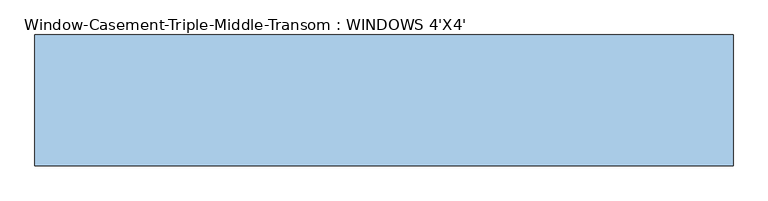
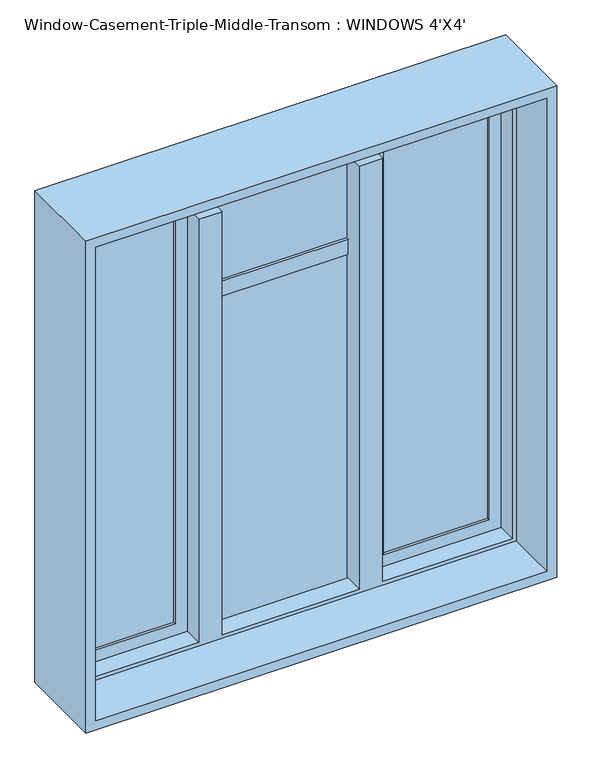
"""IFC4 building model written with IfcOpenShell, lengths in millimetres: window geometry, Window-Casement-Triple-Middle-Transom : WINDOWS 4'X4'."""

from ifc_helpers import new_model, si_unit, frame, origin, place, context, project, spatial, polyline, outline, extrude, faceted_brep, source, transform, mapped, element, save


def window_casement_triple_middle_transom_windows_4_x4_273a115f(model_context):
    return source(origin(), model_context, "Body", "SolidModel", [
        extrude(outline(polyline([(2235.2, 228.6), (939.8, 228.6), (939.8, 584.2), (2235.2, 584.2), (2235.2, 228.6)]), holes=[polyline([(2193.3296875, 542.3296875), (981.6703125, 542.3296875), (981.6703125, 270.4703125), (2193.3296875, 270.4703125), (2193.3296875, 542.3296875)])]), frame((0.0, 73.025, 0.0), z_axis=(0.0, 1.0, 0.0), x_axis=(0.0, 0.0, 1.0)), (0.0, 0.0, 1.0), 31.75),
        extrude(outline(polyline([(2235.2, -584.2), (939.8, -584.2), (939.8, -228.6), (2235.2, -228.6), (2235.2, -584.2)]), holes=[polyline([(2193.3296875, -270.4703125), (981.6703125, -270.4703125), (981.6703125, -542.3296875), (2193.3296875, -542.3296875), (2193.3296875, -270.4703125)])]), frame((0.0, 73.025, 0.0), z_axis=(0.0, 1.0, 0.0), x_axis=(0.0, 0.0, 1.0)), (0.0, 0.0, 1.0), 31.75),
        extrude(outline(polyline([(-270.4703125, 98.425), (-270.4703125, 92.075), (-542.3296875, 92.075), (-542.3296875, 98.425), (-270.4703125, 98.425)])), frame((0.0, 0.0, 949.9203125), z_axis=(0.0, 0.0, 1.0), x_axis=(1.0, 0.0, 0.0)), (0.0, 0.0, 1.0), 1275.159375),
        extrude(outline(polyline([(-270.4703125, 85.725), (-270.4703125, 79.375), (-542.3296875, 79.375), (-542.3296875, 85.725), (-270.4703125, 85.725)])), frame((0.0, 0.0, 949.9203125), z_axis=(0.0, 0.0, 1.0), x_axis=(1.0, 0.0, 0.0)), (0.0, 0.0, 1.0), 1275.159375),
        extrude(outline(polyline([(542.3296875, 98.425), (542.3296875, 92.075), (270.4703125, 92.075), (270.4703125, 98.425), (542.3296875, 98.425)])), frame((0.0, 0.0, 949.9203125), z_axis=(0.0, 0.0, 1.0), x_axis=(1.0, 0.0, 0.0)), (0.0, 0.0, 1.0), 1275.159375),
        extrude(outline(polyline([(542.3296875, 85.725), (542.3296875, 79.375), (270.4703125, 79.375), (270.4703125, 85.725), (542.3296875, 85.725)])), frame((0.0, 0.0, 949.9203125), z_axis=(0.0, 0.0, 1.0), x_axis=(1.0, 0.0, 0.0)), (0.0, 0.0, 1.0), 1275.159375),
        extrude(outline(polyline([(177.8, 104.775), (177.8, 73.025), (-177.8, 73.025), (-177.8, 104.775), (177.8, 104.775)])), frame((0.0, 0.0, 1835.8048438), z_axis=(0.0, 0.0, 1.0), x_axis=(1.0, 0.0, 0.0)), (0.0, 0.0, 1.0), 41.8703125),
        extrude(outline(polyline([(177.8, 98.425), (177.8, 92.075), (-177.8, 92.075), (-177.8, 98.425), (177.8, 98.425)])), frame((0.0, 0.0, 939.8), z_axis=(0.0, 0.0, 1.0), x_axis=(1.0, 0.0, 0.0)), (0.0, 0.0, 1.0), 896.0048437),
        extrude(outline(polyline([(177.8, 85.725), (177.8, 79.375), (-177.8, 79.375), (-177.8, 85.725), (177.8, 85.725)])), frame((0.0, 0.0, 939.8), z_axis=(0.0, 0.0, 1.0), x_axis=(1.0, 0.0, 0.0)), (0.0, 0.0, 1.0), 896.0048437),
        extrude(outline(polyline([(177.8, 98.425), (177.8, 92.075), (-177.8, 92.075), (-177.8, 98.425), (177.8, 98.425)])), frame((0.0, 0.0, 1877.6751563), z_axis=(0.0, 0.0, 1.0), x_axis=(1.0, 0.0, 0.0)), (0.0, 0.0, 1.0), 357.5248438),
        extrude(outline(polyline([(177.8, 85.725), (177.8, 79.375), (-177.8, 79.375), (-177.8, 85.725), (177.8, 85.725)])), frame((0.0, 0.0, 1877.6751563), z_axis=(0.0, 0.0, 1.0), x_axis=(1.0, 0.0, 0.0)), (0.0, 0.0, 1.0), 357.5248438),
        faceted_brep([(-584.2, 73.025, 2235.2), (-584.2, 114.3, 2235.2), (584.2, 114.3, 2235.2), (584.2, 73.025, 2235.2), (-574.0796875, 22.225, 2225.0796875), (-574.0796875, 73.025, 2225.0796875), (574.0796875, 73.025, 2225.0796875), (574.0796875, 22.225, 2225.0796875), (-584.2, -114.3, 2235.2), (-584.2, 22.225, 2235.2), (584.2, 22.225, 2235.2), (584.2, -114.3, 2235.2), (-609.6, 114.3, 2260.6), (-609.6, -114.3, 2260.6), (609.6, -114.3, 2260.6), (609.6, 114.3, 2260.6), (584.2, 114.3, 939.8), (584.2, 73.025, 939.8), (574.0796875, 73.025, 949.9203125), (574.0796875, 22.225, 949.9203125), (584.2, 22.225, 939.8), (584.2, -114.3, 939.8), (609.6, -114.3, 914.4), (609.6, 114.3, 914.4), (228.6, 73.025, 939.8), (-584.2, 114.3, 939.8), (-584.2, 73.025, 939.8), (-228.6, 73.025, 939.8), (-228.6, 111.125, 939.8), (-177.8, 111.125, 939.8), (-177.8, 73.025, 939.8), (177.8, 73.025, 939.8), (177.8, 111.125, 939.8), (228.6, 111.125, 939.8), (238.7203125, 73.025, 949.9203125), (238.7203125, 22.225, 949.9203125), (-574.0796875, 73.025, 949.9203125), (-574.0796875, 22.225, 949.9203125), (-238.7203125, 22.225, 949.9203125), (-238.7203125, 73.025, 949.9203125), (177.8, 73.025, 949.9203125), (-177.8, 73.025, 949.9203125), (-177.8, 22.225, 949.9203125), (177.8, 22.225, 949.9203125), (-584.2, 22.225, 939.8), (-584.2, -114.3, 939.8), (-609.6, -114.3, 914.4), (-609.6, 114.3, 914.4), (228.6, 73.025, 2108.2), (238.7203125, 73.025, 2108.2), (-238.7203125, 73.025, 2108.2), (-228.6, 73.025, 2108.2), (-177.8, 111.125, 2108.2), (-228.6, 111.125, 2108.2), (-238.7203125, 22.225, 2108.2), (-177.8, 22.225, 2108.2), (228.6, 111.125, 2108.2), (177.8, 111.125, 2108.2), (177.8, 22.225, 2108.2), (238.7203125, 22.225, 2108.2)], [[[0, 1, 2, 3]], [[4, 5, 6, 7]], [[8, 9, 10, 11]], [[12, 13, 14, 15]], [[3, 2, 16, 17]], [[7, 6, 18, 19]], [[11, 10, 20, 21]], [[15, 14, 22, 23]], [[24, 17, 16, 25, 26, 27, 28, 29, 30, 31, 32, 33]], [[19, 18, 34, 35]], [[36, 37, 38, 39]], [[40, 41, 42, 43]], [[21, 20, 44, 45]], [[23, 22, 46, 47]], [[1, 0, 26, 25]], [[0, 3, 17, 24, 48, 49, 34, 18, 6, 5, 36, 39, 50, 51, 27, 26]], [[41, 40, 31, 30]], [[5, 4, 37, 36]], [[9, 8, 45, 44]], [[14, 13, 46, 22], [8, 11, 21, 45]], [[13, 12, 47, 46]], [[12, 15, 23, 47], [2, 1, 25, 16]], [[52, 53, 51, 50, 54, 55]], [[56, 57, 58, 59, 49, 48]], [[53, 52, 29, 28]], [[27, 51, 53, 28]], [[52, 55, 42, 41, 30, 29]], [[57, 56, 33, 32]], [[58, 57, 32, 31, 40, 43]], [[56, 48, 24, 33]], [[54, 50, 39, 38]], [[49, 59, 35, 34]], [[10, 9, 44, 20], [4, 7, 19, 35, 59, 58, 43, 42, 55, 54, 38, 37]]]),
    ])


if __name__ == "__main__":
    model = new_model("IFC4")
    model_context = context("Model", 3, world=origin())
    ifc_project = project(units=[si_unit("LENGTHUNIT", "METRE", prefix="MILLI")], contexts=[model_context])
    site = spatial("IfcSite", under=ifc_project)
    building = spatial("IfcBuilding", under=site)
    placement = place(None, origin())
    window_casement_triple_middle_transom_windows_4_x4_shape = window_casement_triple_middle_transom_windows_4_x4_273a115f(model_context)
    element("IfcWindow", 1, ObjectType="Window-Casement-Triple-Middle-Transom : WINDOWS 4'X4'", at=placement, inside=building, context=model_context, shape_type="MappedRepresentation", body=[
        mapped(window_casement_triple_middle_transom_windows_4_x4_shape, transform((0.0, 0.0, 0.0), x_axis=(1.0, 0.0, 0.0), y_axis=(0.0, 1.0, 0.0), z_axis=(0.0, 0.0, 1.0))),
    ])
    save(model, "model.ifc")

# Revit data of these elements
# Type "Window-Casement-Triple-Middle-Transom : WINDOWS 4'X4'"
#   Type Mark = "21"
#   Fire Rating = "0.5h"
#   Assembly Code = "B2020100"
#   Analytic Construction = "Double glazing - domestic"
#   Window Width = 1' - 4"
#   Window Inset [instance default] = 0' - 0 5/8"
#   Wall Thickness [instance default] = 0' - 6"
#   Visual Light Transmittance = 0.81
#   Transom Height Ratio = 0.3
#   Thermal Resistance (R) = 1.8146 (h·ft²·°F)/BTU
#   Solar Heat Gain Coefficient = 0.76
#   Rough Width = 4' - 0 1/2"
#   Rough Height = 4' - 5 1/2"
#   Heat Transfer Coefficient (U) = 0.5511 BTU/(h·ft²·°F)
#   Height = 4' - 5"
#   Transom Height = 1' - 3.9"
#   Frame Gap 3 [instance default] = 0' - 1 83/128"
#   Frame Gap 2 [instance default] = 0' - 0 5/8"
#   Frame Gap 1 = 0' - 1 51/128"
#   Default Sill Height = 3' - 0"
#   Width = 4' - 0"
#   Frame Material = Metal - Aluminum
#   Glass Panel Material = Glass
#   Wall Closure = (empty or 0)
# Element 1 (IfcWindow, "Window-Casement-Triple-Middle-Transom : WINDOWS 4'X4'")
#   Wall Thickness = 0' - 9"
#   Materials on its faces: "Metal - Aluminum", "Glass"
# Materials
#   "Metal - Aluminum": class "Metal", colour RGB 247 247 247, transparency 0, Cost = 0
#   "Glass": class "Glass", colour RGB 0 128 192, transparency 0.75, Description = "Soda Lime Glass", Cost = 0
